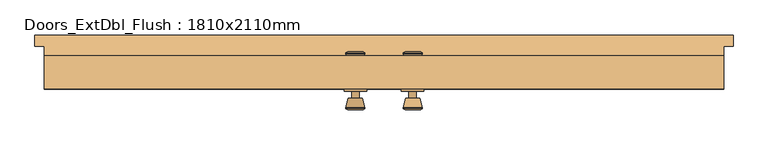
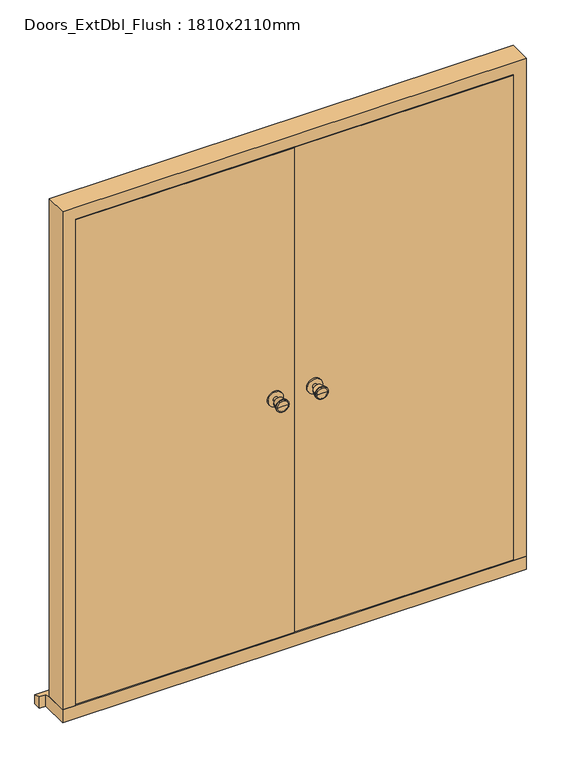
"""IFC4 building model written with IfcOpenShell, lengths in millimetres: door geometry, Doors_ExtDbl_Flush : 1810x2110mm."""

from ifc_helpers import new_model, si_unit, point, frame, frame_2d, origin, place, context, project, spatial, polyline, circle_curve, trimmed, segment, composite_curve, outline, extrude, faceted_brep, source, transform, mapped, element, save
from ifc_brep_helpers import plane_surface, cylinder_surface, revolved_surface, advanced_brep


def doors_extdbl_flush_1810x2110mm_47ab578d(model_context):
    return source(origin(), model_context, "Body", "SolidModel", [
        advanced_brep(
        [(-76.5, -56.4492, 1050.0), (-66.5, -56.4492, 1050.0), (-86.5, -56.4492, 1050.0), (-96.9758676, -105.4492, 1050.0), (-56.0241324, -105.4492, 1050.0), (-76.5, -105.4492, 1050.0), (-101.5, -103.6213319, 1050.0), (-51.5, -103.6213319, 1050.0), (-101.5, -100.1576537, 1050.0), (-51.5, -100.1576537, 1050.0), (-95.136236, -75.4492, 1050.0), (-57.863764, -75.4492, 1050.0), (-86.5, -75.4492, 1050.0), (-66.5, -75.4492, 1050.0)],
        [
            (0, 1),
            (1, 2, circle_curve(frame((-76.5, -56.4492, 1050.0), z_axis=(0.0, 1.0, 0.0), x_axis=(1.0, 0.0, 0.0)), 10.0)),
            (2, 0),
            (2, 1, circle_curve(frame((-76.5, -56.4492, 1050.0), z_axis=(0.0, 1.0, 0.0), x_axis=(1.0, 0.0, 0.0)), 10.0)),
            (3, 4, circle_curve(frame((-76.5, -105.4492, 1050.0), z_axis=(0.0, -1.0, 0.0), x_axis=(1.0, 0.0, 0.0)), 20.4758676)),
            (4, 5),
            (5, 3),
            (4, 3, circle_curve(frame((-76.5, -105.4492, 1050.0), z_axis=(0.0, -1.0, 0.0), x_axis=(1.0, 0.0, 0.0)), 20.4758676)),
            (6, 7, circle_curve(frame((-76.5, -103.6213319, 1050.0), z_axis=(0.0, -1.0, 0.0), x_axis=(1.0, 0.0, 0.0)), 25.0)),
            (7, 4),
            (3, 6),
            (7, 6, circle_curve(frame((-76.5, -103.6213319, 1050.0), z_axis=(0.0, -1.0, 0.0), x_axis=(1.0, 0.0, 0.0)), 25.0)),
            (8, 9, circle_curve(frame((-76.5, -100.1576537, 1050.0), z_axis=(0.0, -1.0, 0.0), x_axis=(1.0, 0.0, 0.0)), 25.0)),
            (9, 7),
            (6, 8),
            (9, 8, circle_curve(frame((-76.5, -100.1576537, 1050.0), z_axis=(0.0, -1.0, 0.0), x_axis=(1.0, 0.0, 0.0)), 25.0)),
            (10, 11, circle_curve(frame((-76.5, -75.4492, 1050.0), z_axis=(0.0, -1.0, 0.0), x_axis=(1.0, 0.0, 0.0)), 18.636236)),
            (11, 9),
            (8, 10),
            (11, 10, circle_curve(frame((-76.5, -75.4492, 1050.0), z_axis=(0.0, -1.0, 0.0), x_axis=(1.0, 0.0, 0.0)), 18.636236)),
            (12, 13, circle_curve(frame((-76.5, -75.4492, 1050.0), z_axis=(0.0, -1.0, 0.0), x_axis=(1.0, 0.0, 0.0)), 10.0)),
            (13, 11),
            (10, 12),
            (13, 12, circle_curve(frame((-76.5, -75.4492, 1050.0), z_axis=(0.0, -1.0, 0.0), x_axis=(1.0, 0.0, 0.0)), 10.0)),
            (1, 13),
            (12, 2),
        ],
        [
            plane_surface(frame((-76.5, -56.4492, 1050.0), z_axis=(0.0, 1.0, 0.0), x_axis=(1.0, 0.0, 0.0))),
            plane_surface(frame((-76.5, -105.4492, 1050.0), z_axis=(0.0, -1.0, 0.0), x_axis=(1.0, 0.0, 0.0))),
            revolved_surface(polyline([(-56.0241324, -105.4492, 1050.0), (-51.5, -103.6213319, 1050.0)]), (-76.5, -56.4492, 1050.0), (0.0, 1.0, 0.0)),
            cylinder_surface(frame((-76.5, -56.4492, 1050.0), z_axis=(0.0, 1.0, 0.0), x_axis=(1.0, 0.0, 0.0)), 25.0),
            revolved_surface(polyline([(-51.5, -100.1576537, 1050.0), (-57.863764, -75.4492, 1050.0)]), (-76.5, -56.4492, 1050.0), (0.0, 1.0, 0.0)),
            plane_surface(frame((-76.5, -75.4492, 1050.0), z_axis=(0.0, 1.0, 0.0), x_axis=(1.0, 0.0, 0.0))),
            cylinder_surface(frame((-76.5, -56.4492, 1050.0), z_axis=(0.0, 1.0, 0.0), x_axis=(1.0, 0.0, 0.0)), 10.0),
        ],
        [
            (0, [[1, 2, 3]]),
            (0, [[-3, 4, -1]]),
            (1, [[5, 6, 7]]),
            (1, [[8, -7, -6]]),
            (2, [[9, 10, -5, 11]]),
            (2, [[12, -11, -8, -10]]),
            (3, [[13, 14, -9, 15]]),
            (3, [[16, -15, -12, -14]]),
            (4, [[17, 18, -13, 19]]),
            (4, [[20, -19, -16, -18]]),
            (5, [[21, 22, -17, 23]]),
            (5, [[24, -23, -20, -22]]),
            (6, [[-2, 25, -21, 26]]),
            (6, [[-4, -26, -24, -25]]),
        ],
    ),
        extrude(outline(composite_curve([segment(trimmed(circle_curve(frame_2d((1050.0, -76.5)), 30.0), [point((1050.0, -46.5))], [point((1050.0, -106.5))], False, "CARTESIAN"), True, "CONTINUOUS"), segment(trimmed(circle_curve(frame_2d((1050.0, -76.5)), 30.0), [point((1050.0, -106.5))], [point((1050.0, -46.5))], False, "CARTESIAN"), True, "CONTINUOUS")], self_intersect=False)), frame((0.0, -56.4492, 0.0), z_axis=(0.0, 1.0, 0.0), x_axis=(0.0, 0.0, 1.0)), (0.0, 0.0, 1.0), 6.0),
        advanced_brep(
        [(-76.5, -0.4492, 1050.0), (-86.5, -0.4492, 1050.0), (-66.5, -0.4492, 1050.0), (-96.9758676, 48.5508, 1050.0), (-76.5, 48.5508, 1050.0), (-56.0241324, 48.5508, 1050.0), (-101.5, 46.7229319, 1050.0), (-51.5, 46.7229319, 1050.0), (-101.5, 43.2592537, 1050.0), (-51.5, 43.2592537, 1050.0), (-95.136236, 18.5508, 1050.0), (-57.863764, 18.5508, 1050.0), (-86.5, 18.5508, 1050.0), (-66.5, 18.5508, 1050.0)],
        [
            (0, 1),
            (1, 2, circle_curve(frame((-76.5, -0.4492, 1050.0), z_axis=(0.0, -1.0, 0.0), x_axis=(1.0, 0.0, 0.0)), 10.0)),
            (2, 0),
            (2, 1, circle_curve(frame((-76.5, -0.4492, 1050.0), z_axis=(0.0, -1.0, 0.0), x_axis=(1.0, 0.0, 0.0)), 10.0)),
            (3, 4),
            (4, 5),
            (5, 3, circle_curve(frame((-76.5, 48.5508, 1050.0), z_axis=(0.0, 1.0, 0.0), x_axis=(1.0, 0.0, 0.0)), 20.4758676)),
            (3, 5, circle_curve(frame((-76.5, 48.5508, 1050.0), z_axis=(0.0, 1.0, 0.0), x_axis=(1.0, 0.0, 0.0)), 20.4758676)),
            (6, 3),
            (5, 7),
            (7, 6, circle_curve(frame((-76.5, 46.7229319, 1050.0), z_axis=(0.0, 1.0, 0.0), x_axis=(1.0, 0.0, 0.0)), 25.0)),
            (6, 7, circle_curve(frame((-76.5, 46.7229319, 1050.0), z_axis=(0.0, 1.0, 0.0), x_axis=(1.0, 0.0, 0.0)), 25.0)),
            (8, 6),
            (7, 9),
            (9, 8, circle_curve(frame((-76.5, 43.2592537, 1050.0), z_axis=(0.0, 1.0, 0.0), x_axis=(1.0, 0.0, 0.0)), 25.0)),
            (8, 9, circle_curve(frame((-76.5, 43.2592537, 1050.0), z_axis=(0.0, 1.0, 0.0), x_axis=(1.0, 0.0, 0.0)), 25.0)),
            (10, 8),
            (9, 11),
            (11, 10, circle_curve(frame((-76.5, 18.5508, 1050.0), z_axis=(0.0, 1.0, 0.0), x_axis=(1.0, 0.0, 0.0)), 18.636236)),
            (10, 11, circle_curve(frame((-76.5, 18.5508, 1050.0), z_axis=(0.0, 1.0, 0.0), x_axis=(1.0, 0.0, 0.0)), 18.636236)),
            (12, 10),
            (11, 13),
            (13, 12, circle_curve(frame((-76.5, 18.5508, 1050.0), z_axis=(0.0, 1.0, 0.0), x_axis=(1.0, 0.0, 0.0)), 10.0)),
            (12, 13, circle_curve(frame((-76.5, 18.5508, 1050.0), z_axis=(0.0, 1.0, 0.0), x_axis=(1.0, 0.0, 0.0)), 10.0)),
            (1, 12),
            (13, 2),
        ],
        [
            plane_surface(frame((-76.5, -0.4492, 1050.0), z_axis=(0.0, -1.0, 0.0), x_axis=(1.0, 0.0, 0.0))),
            plane_surface(frame((-76.5, 48.5508, 1050.0), z_axis=(0.0, 1.0, 0.0), x_axis=(1.0, 0.0, 0.0))),
            revolved_surface(polyline([(-56.0241324, 48.5508, 1050.0), (-51.5, 46.7229319, 1050.0)]), (-76.5, -0.4492, 1050.0), (0.0, -1.0, 0.0)),
            cylinder_surface(frame((-76.5, -0.4492, 1050.0), z_axis=(0.0, -1.0, 0.0), x_axis=(1.0, 0.0, 0.0)), 25.0),
            revolved_surface(polyline([(-51.5, 43.2592537, 1050.0), (-57.863764, 18.5508, 1050.0)]), (-76.5, -0.4492, 1050.0), (0.0, -1.0, 0.0)),
            plane_surface(frame((-76.5, 18.5508, 1050.0), z_axis=(0.0, -1.0, 0.0), x_axis=(1.0, 0.0, 0.0))),
            cylinder_surface(frame((-76.5, -0.4492, 1050.0), z_axis=(0.0, -1.0, 0.0), x_axis=(1.0, 0.0, 0.0)), 10.0),
        ],
        [
            (0, [[1, 2, 3]]),
            (0, [[-3, 4, -1]]),
            (1, [[5, 6, 7]]),
            (1, [[-6, -5, 8]]),
            (2, [[9, -7, 10, 11]]),
            (2, [[-10, -8, -9, 12]]),
            (3, [[13, -11, 14, 15]]),
            (3, [[-14, -12, -13, 16]]),
            (4, [[17, -15, 18, 19]]),
            (4, [[-18, -16, -17, 20]]),
            (5, [[21, -19, 22, 23]]),
            (5, [[-22, -20, -21, 24]]),
            (6, [[25, -23, 26, -2]]),
            (6, [[-26, -24, -25, -4]]),
        ],
    ),
        extrude(outline(composite_curve([segment(trimmed(circle_curve(frame_2d((1050.0, -76.5)), 30.0), [point((1050.0, -46.5))], [point((1050.0, -106.5))], False, "CARTESIAN"), True, "CONTINUOUS"), segment(trimmed(circle_curve(frame_2d((1050.0, -76.5)), 30.0), [point((1050.0, -106.5))], [point((1050.0, -46.5))], False, "CARTESIAN"), True, "CONTINUOUS")], self_intersect=False)), frame((0.0, -6.4492, 0.0), z_axis=(0.0, 1.0, 0.0), x_axis=(0.0, 0.0, 1.0)), (0.0, 0.0, 1.0), 6.0),
        advanced_brep(
        [(76.5, -56.4492, 1050.0), (86.5, -56.4492, 1050.0), (66.5, -56.4492, 1050.0), (96.9758676, -105.4492, 1050.0), (76.5, -105.4492, 1050.0), (56.0241324, -105.4492, 1050.0), (101.5, -103.6213319, 1050.0), (51.5, -103.6213319, 1050.0), (101.5, -100.1576537, 1050.0), (51.5, -100.1576537, 1050.0), (95.136236, -75.4492, 1050.0), (57.863764, -75.4492, 1050.0), (86.5, -75.4492, 1050.0), (66.5, -75.4492, 1050.0)],
        [
            (0, 1),
            (1, 2, circle_curve(frame((76.5, -56.4492, 1050.0), z_axis=(0.0, 1.0, 0.0), x_axis=(-1.0, 0.0, 0.0)), 10.0)),
            (2, 0),
            (2, 1, circle_curve(frame((76.5, -56.4492, 1050.0), z_axis=(0.0, 1.0, 0.0), x_axis=(-1.0, 0.0, 0.0)), 10.0)),
            (3, 4),
            (4, 5),
            (5, 3, circle_curve(frame((76.5, -105.4492, 1050.0), z_axis=(0.0, -1.0, 0.0), x_axis=(-1.0, 0.0, 0.0)), 20.4758676)),
            (3, 5, circle_curve(frame((76.5, -105.4492, 1050.0), z_axis=(0.0, -1.0, 0.0), x_axis=(-1.0, 0.0, 0.0)), 20.4758676)),
            (6, 3),
            (5, 7),
            (7, 6, circle_curve(frame((76.5, -103.6213319, 1050.0), z_axis=(0.0, -1.0, 0.0), x_axis=(-1.0, 0.0, 0.0)), 25.0)),
            (6, 7, circle_curve(frame((76.5, -103.6213319, 1050.0), z_axis=(0.0, -1.0, 0.0), x_axis=(-1.0, 0.0, 0.0)), 25.0)),
            (8, 6),
            (7, 9),
            (9, 8, circle_curve(frame((76.5, -100.1576537, 1050.0), z_axis=(0.0, -1.0, 0.0), x_axis=(-1.0, 0.0, 0.0)), 25.0)),
            (8, 9, circle_curve(frame((76.5, -100.1576537, 1050.0), z_axis=(0.0, -1.0, 0.0), x_axis=(-1.0, 0.0, 0.0)), 25.0)),
            (10, 8),
            (9, 11),
            (11, 10, circle_curve(frame((76.5, -75.4492, 1050.0), z_axis=(0.0, -1.0, 0.0), x_axis=(-1.0, 0.0, 0.0)), 18.636236)),
            (10, 11, circle_curve(frame((76.5, -75.4492, 1050.0), z_axis=(0.0, -1.0, 0.0), x_axis=(-1.0, 0.0, 0.0)), 18.636236)),
            (12, 10),
            (11, 13),
            (13, 12, circle_curve(frame((76.5, -75.4492, 1050.0), z_axis=(0.0, -1.0, 0.0), x_axis=(-1.0, 0.0, 0.0)), 10.0)),
            (12, 13, circle_curve(frame((76.5, -75.4492, 1050.0), z_axis=(0.0, -1.0, 0.0), x_axis=(-1.0, 0.0, 0.0)), 10.0)),
            (1, 12),
            (13, 2),
        ],
        [
            plane_surface(frame((76.5, -56.4492, 1050.0), z_axis=(0.0, 1.0, 0.0), x_axis=(-1.0, 0.0, 0.0))),
            plane_surface(frame((76.5, -105.4492, 1050.0), z_axis=(0.0, -1.0, 0.0), x_axis=(-1.0, 0.0, 0.0))),
            revolved_surface(polyline([(56.0241324, -105.4492, 1050.0), (51.5, -103.6213319, 1050.0)]), (76.5, -56.4492, 1050.0), (0.0, 1.0, 0.0)),
            cylinder_surface(frame((76.5, -56.4492, 1050.0), z_axis=(0.0, 1.0, 0.0), x_axis=(-1.0, 0.0, 0.0)), 25.0),
            revolved_surface(polyline([(51.5, -100.1576537, 1050.0), (57.863764, -75.4492, 1050.0)]), (76.5, -56.4492, 1050.0), (0.0, 1.0, 0.0)),
            plane_surface(frame((76.5, -75.4492, 1050.0), z_axis=(0.0, 1.0, 0.0), x_axis=(-1.0, 0.0, 0.0))),
            cylinder_surface(frame((76.5, -56.4492, 1050.0), z_axis=(0.0, 1.0, 0.0), x_axis=(-1.0, 0.0, 0.0)), 10.0),
        ],
        [
            (0, [[1, 2, 3]]),
            (0, [[-3, 4, -1]]),
            (1, [[5, 6, 7]]),
            (1, [[-6, -5, 8]]),
            (2, [[9, -7, 10, 11]]),
            (2, [[-10, -8, -9, 12]]),
            (3, [[13, -11, 14, 15]]),
            (3, [[-14, -12, -13, 16]]),
            (4, [[17, -15, 18, 19]]),
            (4, [[-18, -16, -17, 20]]),
            (5, [[21, -19, 22, 23]]),
            (5, [[-22, -20, -21, 24]]),
            (6, [[25, -23, 26, -2]]),
            (6, [[-26, -24, -25, -4]]),
        ],
    ),
        extrude(outline(composite_curve([segment(trimmed(circle_curve(frame_2d((1050.0, 76.5)), 30.0), [point((1050.0, 46.5))], [point((1050.0, 106.5))], False, "CARTESIAN"), True, "CONTINUOUS"), segment(trimmed(circle_curve(frame_2d((1050.0, 76.5)), 30.0), [point((1050.0, 106.5))], [point((1050.0, 46.5))], False, "CARTESIAN"), True, "CONTINUOUS")], self_intersect=False)), frame((0.0, -56.4492, 0.0), z_axis=(0.0, 1.0, 0.0), x_axis=(0.0, 0.0, 1.0)), (0.0, 0.0, 1.0), 6.0),
        advanced_brep(
        [(76.5, -0.4492, 1050.0), (66.5, -0.4492, 1050.0), (86.5, -0.4492, 1050.0), (96.9758676, 48.5508, 1050.0), (56.0241324, 48.5508, 1050.0), (76.5, 48.5508, 1050.0), (101.5, 46.7229319, 1050.0), (51.5, 46.7229319, 1050.0), (101.5, 43.2592537, 1050.0), (51.5, 43.2592537, 1050.0), (95.136236, 18.5508, 1050.0), (57.863764, 18.5508, 1050.0), (86.5, 18.5508, 1050.0), (66.5, 18.5508, 1050.0)],
        [
            (0, 1),
            (1, 2, circle_curve(frame((76.5, -0.4492, 1050.0), z_axis=(0.0, -1.0, 0.0), x_axis=(-1.0, 0.0, 0.0)), 10.0)),
            (2, 0),
            (2, 1, circle_curve(frame((76.5, -0.4492, 1050.0), z_axis=(0.0, -1.0, 0.0), x_axis=(-1.0, 0.0, 0.0)), 10.0)),
            (3, 4, circle_curve(frame((76.5, 48.5508, 1050.0), z_axis=(0.0, 1.0, 0.0), x_axis=(-1.0, 0.0, 0.0)), 20.4758676)),
            (4, 5),
            (5, 3),
            (4, 3, circle_curve(frame((76.5, 48.5508, 1050.0), z_axis=(0.0, 1.0, 0.0), x_axis=(-1.0, 0.0, 0.0)), 20.4758676)),
            (6, 7, circle_curve(frame((76.5, 46.7229319, 1050.0), z_axis=(0.0, 1.0, 0.0), x_axis=(-1.0, 0.0, 0.0)), 25.0)),
            (7, 4),
            (3, 6),
            (7, 6, circle_curve(frame((76.5, 46.7229319, 1050.0), z_axis=(0.0, 1.0, 0.0), x_axis=(-1.0, 0.0, 0.0)), 25.0)),
            (8, 9, circle_curve(frame((76.5, 43.2592537, 1050.0), z_axis=(0.0, 1.0, 0.0), x_axis=(-1.0, 0.0, 0.0)), 25.0)),
            (9, 7),
            (6, 8),
            (9, 8, circle_curve(frame((76.5, 43.2592537, 1050.0), z_axis=(0.0, 1.0, 0.0), x_axis=(-1.0, 0.0, 0.0)), 25.0)),
            (10, 11, circle_curve(frame((76.5, 18.5508, 1050.0), z_axis=(0.0, 1.0, 0.0), x_axis=(-1.0, 0.0, 0.0)), 18.636236)),
            (11, 9),
            (8, 10),
            (11, 10, circle_curve(frame((76.5, 18.5508, 1050.0), z_axis=(0.0, 1.0, 0.0), x_axis=(-1.0, 0.0, 0.0)), 18.636236)),
            (12, 13, circle_curve(frame((76.5, 18.5508, 1050.0), z_axis=(0.0, 1.0, 0.0), x_axis=(-1.0, 0.0, 0.0)), 10.0)),
            (13, 11),
            (10, 12),
            (13, 12, circle_curve(frame((76.5, 18.5508, 1050.0), z_axis=(0.0, 1.0, 0.0), x_axis=(-1.0, 0.0, 0.0)), 10.0)),
            (1, 13),
            (12, 2),
        ],
        [
            plane_surface(frame((76.5, -0.4492, 1050.0), z_axis=(0.0, -1.0, 0.0), x_axis=(-1.0, 0.0, 0.0))),
            plane_surface(frame((76.5, 48.5508, 1050.0), z_axis=(0.0, 1.0, 0.0), x_axis=(-1.0, 0.0, 0.0))),
            revolved_surface(polyline([(56.0241324, 48.5508, 1050.0), (51.5, 46.7229319, 1050.0)]), (76.5, -0.4492, 1050.0), (0.0, -1.0, 0.0)),
            cylinder_surface(frame((76.5, -0.4492, 1050.0), z_axis=(0.0, -1.0, 0.0), x_axis=(-1.0, 0.0, 0.0)), 25.0),
            revolved_surface(polyline([(51.5, 43.2592537, 1050.0), (57.863764, 18.5508, 1050.0)]), (76.5, -0.4492, 1050.0), (0.0, -1.0, 0.0)),
            plane_surface(frame((76.5, 18.5508, 1050.0), z_axis=(0.0, -1.0, 0.0), x_axis=(-1.0, 0.0, 0.0))),
            cylinder_surface(frame((76.5, -0.4492, 1050.0), z_axis=(0.0, -1.0, 0.0), x_axis=(-1.0, 0.0, 0.0)), 10.0),
        ],
        [
            (0, [[1, 2, 3]]),
            (0, [[-3, 4, -1]]),
            (1, [[5, 6, 7]]),
            (1, [[8, -7, -6]]),
            (2, [[9, 10, -5, 11]]),
            (2, [[12, -11, -8, -10]]),
            (3, [[13, 14, -9, 15]]),
            (3, [[16, -15, -12, -14]]),
            (4, [[17, 18, -13, 19]]),
            (4, [[20, -19, -16, -18]]),
            (5, [[21, 22, -17, 23]]),
            (5, [[24, -23, -20, -22]]),
            (6, [[-2, 25, -21, 26]]),
            (6, [[-4, -26, -24, -25]]),
        ],
    ),
        extrude(outline(composite_curve([segment(trimmed(circle_curve(frame_2d((1050.0, 76.5)), 30.0), [point((1050.0, 46.5))], [point((1050.0, 106.5))], False, "CARTESIAN"), True, "CONTINUOUS"), segment(trimmed(circle_curve(frame_2d((1050.0, 76.5)), 30.0), [point((1050.0, 106.5))], [point((1050.0, 46.5))], False, "CARTESIAN"), True, "CONTINUOUS")], self_intersect=False)), frame((0.0, -6.4492, 0.0), z_axis=(0.0, 1.0, 0.0), x_axis=(0.0, 0.0, 1.0)), (0.0, 0.0, 1.0), 6.0),
        faceted_brep([(834.5, 38.5508, 54.5), (905.0, 38.5508, 54.5), (905.0, -50.4492, 54.5), (856.5, -50.4492, 54.5), (856.5, -3.4492, 54.5), (834.5, -3.4492, 54.5), (834.5, 38.5508, 2039.5), (-834.5, 38.5508, 2039.5), (-834.5, 38.5508, 54.5), (-905.0, 38.5508, 54.5), (-905.0, 38.5508, 2110.0), (905.0, 38.5508, 2110.0), (905.0, -50.4492, 2110.0), (-905.0, -50.4492, 2110.0), (-905.0, -50.4492, 54.5), (-856.5, -50.4492, 54.5), (-856.5, -50.4492, 2061.5), (856.5, -50.4492, 2061.5), (856.5, -3.4492, 2061.5), (-856.5, -3.4492, 2061.5), (-856.5, -3.4492, 54.5), (-834.5, -3.4492, 54.5), (-834.5, -3.4492, 2039.5), (834.5, -3.4492, 2039.5)], [[[0, 1, 2, 3, 4, 5]], [[1, 0, 6, 7, 8, 9, 10, 11]], [[2, 1, 11, 12]], [[3, 2, 12, 13, 14, 15, 16, 17]], [[4, 3, 17, 18]], [[5, 4, 18, 19, 20, 21, 22, 23]], [[0, 5, 23, 6]], [[12, 11, 10, 13]], [[18, 17, 16, 19]], [[6, 23, 22, 7]], [[8, 21, 20, 15, 14, 9]], [[13, 10, 9, 14]], [[19, 16, 15, 20]], [[7, 22, 21, 8]]]),
        faceted_brep([(930.0, 93.5508, 0.0), (930.0, 93.5508, 38.5947221), (930.0, 63.5508, 47.2703282), (930.0, 63.5508, 0.0), (-930.0, 93.5508, 38.5947221), (-930.0, 93.5508, 0.0), (-930.0, 63.5508, 0.0), (-930.0, 63.5508, 47.2703282), (905.0, 63.5508, 0.0), (905.0, -50.4492, 0.0), (-905.0, -50.4492, 0.0), (-905.0, 63.5508, 0.0), (-905.0, 63.5508, 47.2703282), (-905.0, 38.5508, 54.5), (905.0, 38.5508, 54.5), (905.0, 63.5508, 47.2703282), (-905.0, -50.4492, 54.5), (905.0, -50.4492, 54.5)], [[[0, 1, 2, 3]], [[4, 5, 6, 7]], [[5, 0, 3, 8, 9, 10, 11, 6]], [[1, 0, 5, 4]], [[1, 4, 7, 12, 13, 14, 15, 2]], [[13, 16, 17, 14]], [[16, 10, 9, 17]], [[12, 11, 10, 16, 13]], [[11, 12, 7, 6]], [[8, 15, 14, 17, 9]], [[15, 8, 3, 2]]]),
        extrude(outline(polyline([(853.5, -50.4492), (1.5, -50.4492), (1.5, -6.4492), (853.5, -6.4492), (853.5, -50.4492)])), frame((0.0, 0.0, 58.5), z_axis=(0.0, 0.0, 1.0), x_axis=(1.0, 0.0, 0.0)), (0.0, 0.0, 1.0), 2000.0),
        extrude(outline(polyline([(-1.5, -50.4492), (-853.5, -50.4492), (-853.5, -6.4492), (-1.5, -6.4492), (-1.5, -50.4492)])), frame((0.0, 0.0, 58.5), z_axis=(0.0, 0.0, 1.0), x_axis=(1.0, 0.0, 0.0)), (0.0, 0.0, 1.0), 2000.0),
    ])


if __name__ == "__main__":
    model = new_model("IFC4")
    model_context = context("Model", 3, world=origin())
    ifc_project = project(units=[si_unit("LENGTHUNIT", "METRE", prefix="MILLI")], contexts=[model_context])
    site = spatial("IfcSite", under=ifc_project)
    building = spatial("IfcBuilding", under=site)
    placement = place(None, origin())
    doors_extdbl_flush_1810x2110mm_shape = doors_extdbl_flush_1810x2110mm_47ab578d(model_context)
    element("IfcDoor", 1, ObjectType="Doors_ExtDbl_Flush : 1810x2110mm", at=placement, inside=building, context=model_context, shape_type="MappedRepresentation", body=[
        mapped(doors_extdbl_flush_1810x2110mm_shape, transform((0.0, 0.0, 0.0), x_axis=(1.0, 0.0, 0.0), y_axis=(0.0, 1.0, 0.0), z_axis=(0.0, 0.0, 1.0))),
    ])
    save(model, "model.ifc")

# Revit data of these elements
# Type "Doors_ExtDbl_Flush : 1810x2110mm"
#   Type Mark = "44"
#   Type Comments = "External Double"
#   Operation = "DoubleDoorSingleSwing"
#   Keynote = "L20"
#   Analytic Construction = "Metal"
#   Wrap Layers (Ext) from Ext = 102.5 mm
#   Wrap Layers (Int) from Ext = 177.5 mm
#   Thickness = 44 mm
#   Rough Width = 1810 mm
#   Rough Height = 2110 mm
#   O/A Frame Width = 64 mm
#   Heat Transfer Coefficient (U) = 3.7021 W/(m²·K)
#   Handle Z Distance = 1050 mm
#   FrameWidth = 42 mm
#   FrameOffset - External = 25 mm
#   FrameDepth = 89 mm
#   Door Panel Width = 852 mm
#   Door Panel Thickness = 44 mm
#   Door Panel Height = 2000 mm
#   Cill Thickness = 54.5 mm
#   Cill Projection = 30 mm
#   Handle X Distance = 75 mm
#   Height = 2110 mm
#   Structural Tolerance = 6.5 mm
#   Tolerance = 3 mm
#   Undercut = 4 mm
#   Width = 1810 mm
#   Cill Extension = 25 mm
#   Cavity Closer Width = 50 mm
#   Cavity Closer Offset from Ext = 102.5 mm
#   Cavity Closer Depth = 85 mm
#   Define Thermal Properties by = 0
#   Vis - Ironmongery = yes
#   Vis - Cavity Closers = yes
#   Function = 1
#   Material Door = Door - Panel
#   Material Frame = Door - Frame/Mullion
#   Material Ironmongery = Door - Handle
#   Visual Light Transmittance = 0
#   Thermal Resistance (R) = 0
#   Solar Heat Gain Coefficient = 0
#   Wall Closure = (empty or 0)
# Element 1 (IfcDoor, "Doors_ExtDbl_Flush : 1810x2110mm")
#   Materials on its faces: "Door - Handle", "Door - Frame/Mullion", "Door - Panel"
# Materials
#   "Door - Panel": class "Wood", colour RGB 210 159 95, transparency 0, Keynote = "L20", Cost = 0
#   "Door - Frame/Mullion": class "Wood", colour RGB 212 179 113, transparency 0, Keynote = "L20", Cost = 0
#   "Door - Handle": colour RGB 0 0 0, transparency 0, Keynote = "P21", Cost = 0
